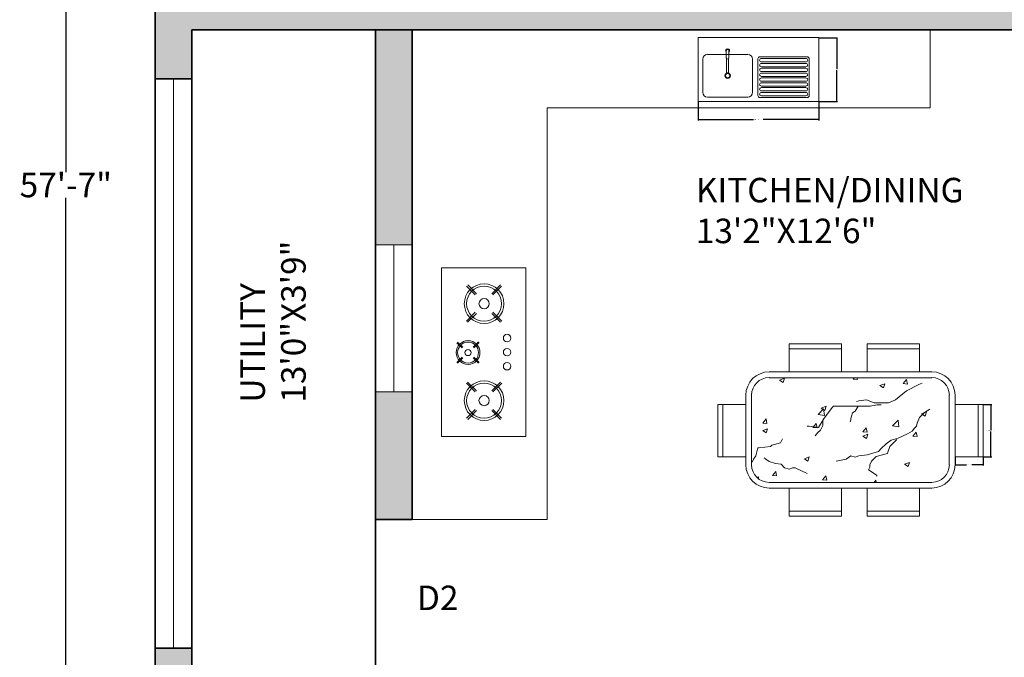
# Model space of a CAD drawing. Units: inches. Extents: x -9 to 505, y -680 to 48.
# Tile 2 of 17: x -6 to 235, y -450 to -293. Entities that reach past the tile are written whole.
import ezdxf

# ---------------------------------------------------------------- set-up
doc = ezdxf.new("R2010")
doc.units = ezdxf.units.IN
doc.header["$MEASUREMENT"] = 0
for name, color, linetype, lineweight in [('A-ANNO-DIMS', 2, 'Continuous', 18), ('A-ANNO-TEXT', 7, 'Continuous', 18), ('A-AREA-IDEN', 7, 'Continuous', 18), ('A-EQPM', 8, 'Continuous', 18), ('A-FLOR-CASE', 8, 'Continuous', 18), ('A-FLOR-FIXT', 9, 'Continuous', 18), ('A-FLOR-HRAL', 4, 'Continuous', 18), ('A-FURN', 8, 'Continuous', 18), ('A-GLAZ', 4, 'Continuous', 18), ('A-WALL', 7, 'Continuous', 35), ('A-WALL-PATT', 251, 'Continuous', 13), ('S-CONC', 7, 'Continuous', 35), ('S-CONC-PATT', 18, 'Continuous', 13)]:
    doc.layers.add(name, color=color, linetype=linetype, lineweight=lineweight)
doc.styles.get("Standard").update_dxf_attribs({"font": 'arial.ttf'})
doc.dimstyles.get("Standard").update_dxf_attribs({"dimtxt": 0.18, "dimasz": 0.18, "dimexe": 0.18, "dimexo": 0.0625, "dimgap": 0.09, "dimtad": 0, "dimtih": 1, "dimtoh": 1, "dimdec": 0, "dimzin": 0, "dimdsep": 46, "dimlunit": 3, "dimtxsty": 'Standard', "dimcen": 0.09, "dimadec": 0, "dimazin": 0, "dimtfac": 1, "dimtdec": 0, "dimtofl": 0, "dimtmove": 0, "dimatfit": 3, "dimfxl": 1, "dimtolj": 1, "dimtzin": 0, "dimarcsym": 0})

# ---------------------------------------------------------------- blocks, each defined once
blk = doc.blocks.new('*D3')
at = {"layer": 'A-ANNO-DIMS', "color": 0, "lineweight": -2, "transparency": 16777216}
for p, q in [((27.2, 11.5), (5.16, 11.5)), ((5.34, 11.32), (5.34, -330.86)), ((5.34, -679.32), (5.34, -337.14)), ((27.2, -679.5), (5.16, -679.5))]:
    blk.add_line(p, q, dxfattribs=at)
at = {"layer": 'A-ANNO-DIMS', "color": 0, "transparency": 16777216}
for points in [[(5.31, 11.32), (5.37, 11.32), (5.34, 11.5)], [(5.31, -679.32), (5.37, -679.32), (5.34, -679.5)]]:
    blk.add_solid(points, dxfattribs=at)
at = {"layer": 'Defpoints', "color": 0, "transparency": 16777216}
for p in [(27.26, 11.5), (5.34, -679.5), (27.26, -679.5)]:
    blk.add_point(p, dxfattribs=at)
at = {"layer": 'A-ANNO-DIMS', "color": 0, "transparency": 16777216, "insert": (5.34, -334), "char_height": 6, "attachment_point": 5}
blk.add_mtext('\\A1;57\'-7"', dxfattribs=at)
blk = doc.blocks.new('WIN-36')
for p, q in [((0, 36), (0, 0)), ((9, 36), (0, 36)), ((4.5, 36), (4.5, 2.23)), ((9, 0), (9, 36)), ((0, 0), (9, 0)), ((4.5, 2.23), (4.5, 0))]:
    blk.add_line(p, q)
blk = doc.blocks.new('SINK-SINGLE-DRAINBOARD')
for p, q in [((0, 0), (0, 15.65)), ((0, 15.65), (29.6, 15.65)), ((29.6, 0), (29.6, 15.65)), ((1.13, 10.39), (1.13, 2.25)), ((7.43, 11.55), (2.3, 11.55)), ((12.19, 11.55), (7.57, 11.55)), ((13.36, 2.25), (13.36, 10.39)), ((14.68, 10.42), (14.68, 1.51)), ((26.71, 10.96), (15.22, 10.96)), ((20.97, 10.52), (15.55, 10.52)), ((20.97, 9.72), (15.55, 9.72)), ((20.97, 10.52), (26.39, 10.52)), ((20.97, 9.72), (26.39, 9.72)), ((27.25, 10.42), (27.25, 1.51)), ((20.97, 9.34), (15.55, 9.34)), ((20.97, 8.53), (15.55, 8.53)), ((20.97, 8.15), (15.55, 8.15)), ((20.97, 7.34), (15.55, 7.34)), ((20.97, 9.34), (26.39, 9.34)), ((20.97, 8.53), (26.39, 8.53)), ((20.97, 8.15), (26.39, 8.15)), ((20.97, 7.34), (26.39, 7.34)), ((20.97, 6.96), (15.55, 6.96)), ((20.97, 6.15), (15.55, 6.15)), ((20.97, 5.77), (15.55, 5.77)), ((20.97, 4.96), (15.55, 4.96)), ((20.97, 6.96), (26.39, 6.96)), ((20.97, 6.15), (26.39, 6.15)), ((20.97, 5.77), (26.39, 5.77)), ((20.97, 4.96), (26.39, 4.96)), ((20.97, 4.58), (15.55, 4.58)), ((20.97, 3.78), (15.55, 3.78)), ((20.97, 3.4), (15.55, 3.4)), ((20.97, 2.59), (15.55, 2.59)), ((20.97, 4.58), (26.39, 4.58)), ((20.97, 3.78), (26.39, 3.78)), ((20.97, 3.4), (26.39, 3.4)), ((20.97, 2.59), (26.39, 2.59)), ((2.3, 1.09), (12.19, 1.09)), ((15.22, 0.97), (26.71, 0.97)), ((20.97, 2.21), (15.55, 2.21)), ((20.97, 1.4), (15.55, 1.4)), ((20.97, 2.21), (26.39, 2.21)), ((20.97, 1.4), (26.39, 1.4)), ((0, 0), (29.6, 0))]:
    blk.add_line(p, q)
for points in [[(6.92, 12.46), (6.92, 10.68)], [(7.57, 12.46), (7.57, 10.68)], [(7, 10.48), (7, 7.2)], [(7.49, 10.48), (7.49, 7.2)]]:
    blk.add_lwpolyline(points)
for radius in [0.674, 0.54]:
    blk.add_circle((7.25, 6.32), radius)
for centre, radius, start, end in [((7.25, 12.46), 0.485, 311.9018, 228.0982), ((7.25, 12.46), 0.324, 0, 180), ((2.3, 10.39), 1.17, 90, 180), ((7.25, 10.69), 0.324, 182.2198, 357.7802), ((12.19, 10.39), 1.17, 0, 90), ((15.22, 10.42), 0.54, 90, 180), ((15.55, 9.99), 0.54, 90, 165.5097), ((15.55, 10.26), 0.54, 194.4903, 270), ((26.39, 9.99), 0.54, 14.4903, 90), ((26.39, 10.26), 0.54, 270, 345.5097), ((26.71, 10.42), 0.54, 0, 90), ((15.55, 8.8), 0.54, 90, 165.5097), ((15.55, 9.07), 0.54, 194.4903, 270), ((15.55, 7.61), 0.54, 90, 165.5097), ((15.55, 7.88), 0.54, 194.4903, 270), ((26.39, 8.8), 0.54, 14.4903, 90), ((26.39, 9.07), 0.54, 270, 345.5097), ((26.39, 7.61), 0.54, 14.4903, 90), ((26.39, 7.88), 0.54, 270, 345.5097), ((7.25, 7.18), 0.244, 174.9463, 5.0537), ((15.55, 6.42), 0.54, 90, 165.5097), ((15.55, 6.69), 0.54, 194.4903, 270), ((15.55, 5.23), 0.54, 90, 165.5097), ((15.55, 5.5), 0.54, 194.4903, 270), ((26.39, 6.42), 0.54, 14.4903, 90), ((26.39, 6.69), 0.54, 270, 345.5097), ((26.39, 5.23), 0.54, 14.4903, 90), ((26.39, 5.5), 0.54, 270, 345.5097), ((15.55, 4.05), 0.54, 90, 165.5097), ((15.55, 4.32), 0.54, 194.4903, 270), ((15.55, 2.86), 0.54, 90, 165.5097), ((15.55, 3.13), 0.54, 194.4903, 270), ((26.39, 4.05), 0.54, 14.4903, 90), ((26.39, 4.32), 0.54, 270, 345.5097), ((26.39, 2.86), 0.54, 14.4903, 90), ((26.39, 3.13), 0.54, 270, 345.5097), ((2.3, 2.25), 1.17, 180, 270), ((12.19, 2.25), 1.17, 270, 0), ((15.22, 1.51), 0.54, 180, 270), ((15.55, 1.67), 0.54, 90, 165.5097), ((15.55, 1.94), 0.54, 194.4903, 270), ((26.39, 1.67), 0.54, 14.4903, 90), ((26.39, 1.94), 0.54, 270, 345.5097), ((26.71, 1.51), 0.54, 270, 0)]:
    blk.add_arc(centre, radius, start, end)
blk = doc.blocks.new('CHAIR-DINING-RECTANGULAR')
for p, q in [((6.87, 12.83), (0, 12.83)), ((5.62, 12.83), (5.62, 0)), ((6.87, 0), (6.87, 12.83)), ((0, 0), (6.87, 0))]:
    blk.add_line(p, q)
blk = doc.blocks.new('*D28')
at = {"layer": 'A-ANNO-DIMS', "color": 0, "lineweight": -2, "transparency": 16777216}
for p, q in [((160.34, -313.6), (160.34, -318.15)), ((189.94, -313.6), (189.94, -318.15)), ((160.52, -317.97), (173.96, -317.97)), ((189.76, -317.97), (176.32, -317.97))]:
    blk.add_line(p, q, dxfattribs=at)
at = {"layer": 'A-ANNO-DIMS', "color": 0, "transparency": 16777216}
for points in [[(160.52, -317.94), (160.52, -318), (160.34, -317.97)], [(189.76, -317.94), (189.76, -318), (189.94, -317.97)]]:
    blk.add_solid(points, dxfattribs=at)
at = {"layer": 'Defpoints', "color": 0, "transparency": 16777216}
for p in [(160.34, -313.53), (189.94, -313.53), (189.94, -317.97)]:
    blk.add_point(p, dxfattribs=at)
at = {"layer": 'A-ANNO-DIMS', "color": 0, "transparency": 16777216, "insert": (175.14, -317.97), "char_height": 0.18, "attachment_point": 5}
blk.add_mtext('\\A1;SINK 2\'-5 1/2" TYP.', dxfattribs=at)
blk = doc.blocks.new('*D29')
at = {"layer": 'A-ANNO-DIMS', "color": 0, "lineweight": -2, "transparency": 16777216}
for p, q in [((190, -297.89), (194.56, -297.89)), ((194.38, -298.07), (194.38, -305.53)), ((194.38, -313.35), (194.38, -305.89)), ((190, -313.53), (194.56, -313.53))]:
    blk.add_line(p, q, dxfattribs=at)
at = {"layer": 'A-ANNO-DIMS', "color": 0, "transparency": 16777216}
for points in [[(194.35, -298.07), (194.41, -298.07), (194.38, -297.89)], [(194.35, -313.35), (194.41, -313.35), (194.38, -313.53)]]:
    blk.add_solid(points, dxfattribs=at)
at = {"layer": 'Defpoints', "color": 0, "transparency": 16777216}
for p in [(189.94, -297.89), (194.38, -297.89), (189.94, -313.53)]:
    blk.add_point(p, dxfattribs=at)
at = {"layer": 'A-ANNO-DIMS', "color": 0, "transparency": 16777216, "insert": (194.38, -305.71), "char_height": 0.18, "attachment_point": 5}
blk.add_mtext('\\A1;1\'-3 1/2" TYP.', dxfattribs=at)
blk = doc.blocks.new('*D40')
at = {"layer": 'A-ANNO-DIMS', "color": 0, "lineweight": -2, "transparency": 16777216}
for p, q in [((230.29, -387.8), (232.33, -387.8)), ((232.15, -387.98), (232.15, -394.03)), ((232.15, -400.45), (232.15, -394.4)), ((230.29, -400.63), (232.33, -400.63))]:
    blk.add_line(p, q, dxfattribs=at)
at = {"layer": 'A-ANNO-DIMS', "color": 0, "transparency": 16777216}
for points in [[(232.12, -387.98), (232.18, -387.98), (232.15, -387.8)], [(232.12, -400.45), (232.18, -400.45), (232.15, -400.63)]]:
    blk.add_solid(points, dxfattribs=at)
at = {"layer": 'Defpoints', "color": 0, "transparency": 16777216}
for p in [(230.23, -387.8), (232.15, -387.8), (230.23, -400.63)]:
    blk.add_point(p, dxfattribs=at)
at = {"layer": 'A-ANNO-DIMS', "color": 0, "transparency": 16777216, "insert": (232.15, -394.21), "char_height": 0.18, "attachment_point": 5}
blk.add_mtext('\\A1;SIDE CHAIR 1\'-1" TYP.', dxfattribs=at)
blk = doc.blocks.new('*D41')
at = {"layer": 'A-ANNO-DIMS', "color": 0, "lineweight": -2, "transparency": 16777216}
for p, q in [((223.36, -400.69), (223.36, -402.73)), ((230.23, -400.69), (230.23, -402.73)), ((223.54, -402.55), (226.15, -402.55)), ((230.05, -402.55), (227.43, -402.55))]:
    blk.add_line(p, q, dxfattribs=at)
at = {"layer": 'A-ANNO-DIMS', "color": 0, "transparency": 16777216}
for points in [[(223.54, -402.52), (223.54, -402.58), (223.36, -402.55)], [(230.05, -402.52), (230.05, -402.58), (230.23, -402.55)]]:
    blk.add_solid(points, dxfattribs=at)
at = {"layer": 'Defpoints', "color": 0, "transparency": 16777216}
for p in [(223.36, -400.63), (230.23, -400.63), (230.23, -402.55)]:
    blk.add_point(p, dxfattribs=at)
at = {"layer": 'A-ANNO-DIMS', "color": 0, "transparency": 16777216, "insert": (226.79, -402.55), "char_height": 0.18, "attachment_point": 5}
blk.add_mtext('\\A1;0\'-7" TYP.', dxfattribs=at)

msp = doc.modelspace()

# ---------------------------------------------------------------- hatches: boundary and pattern name
at = {"layer": 'A-WALL-PATT'}
h = msp.add_hatch(color=256, dxfattribs=at)
h.dxf.hatch_style = 1
h.paths.add_polyline_path([(101.64, 11.5), (48.26, 11.5), (48.26, 2.5), (72.26, 2.5), (72.26, -21.25), (81.26, -21.25), (81.26, 2.5), (101.64, 2.5)])
h.paths.add_polyline_path([(36.26, 2.5), (27.26, 2.5), (27.26, -6.92), (36.26, -6.92)])
h.paths.add_polyline_path([(81.26, -57.25), (72.26, -57.25), (72.26, -75.5), (81.26, -75.5)])
h.paths.add_polyline_path([(162.76, 11.5), (137.64, 11.5), (137.64, 2.5), (162.76, 2.5)])
h.paths.add_polyline_path([(179.26, 2.5), (174.76, 2.5), (174.76, -75.5), (179.26, -75.5), (179.26, -54.5), (229.51, -54.5), (229.51, -45.5), (179.26, -45.5)])
h.paths.add_polyline_path([(382.26, -45.5), (332.26, -45.5), (332.26, 2.5), (327.76, 2.5), (327.76, -45.5), (277.51, -45.5), (277.51, -54.5), (327.76, -54.5), (327.76, -111.5), (332.26, -111.5), (332.26, -54.5), (382.26, -54.5)])
h.paths.add_polyline_path([(332.26, -128), (327.76, -128), (327.76, -207), (332.26, -207)])
h.paths.add_polyline_path([(124.76, -111.5), (36.26, -111.5), (36.26, -116), (120.26, -116), (120.26, -168.5), (179.26, -168.5), (179.26, -164), (124.76, -164)])
h.paths.add_polyline_path([(96.26, -164), (36.26, -164), (36.26, -152), (27.26, -152), (27.26, -208.88), (36.26, -208.88), (36.26, -168.5), (96.26, -168.5)])
h.paths.add_polyline_path([(36.26, -244.88), (27.26, -244.88), (27.26, -287), (36.26, -287)])
h.paths.add_polyline_path([(179.26, -204.5), (174.76, -204.5), (174.76, -287), (179.26, -287)])
h.paths.add_polyline_path([(257.26, -296), (248.26, -296), (248.26, -446), (269.26, -446), (269.26, -437), (257.26, -437)])
h.paths.add_polyline_path([(90.26, -296), (81.26, -296), (81.26, -348.67), (90.26, -348.67)])
h.paths.add_polyline_path([(90.26, -384.67), (81.26, -384.67), (81.26, -416), (90.26, -416)])
h.paths.add_polyline_path([(170.26, -452), (36.26, -452), (36.26, -456.5), (165.76, -456.5), (165.76, -504.5), (165.13, -504.5), (165.13, -509), (170.26, -509)])
h.paths.add_polyline_path([(141.76, -504.5), (36.26, -504.5), (36.26, -492.5), (27.26, -492.5), (27.26, -565.96), (36.26, -565.96), (36.26, -509), (141.76, -509)])
h.paths.add_polyline_path([(36.26, -601.96), (27.26, -601.96), (27.26, -658.5), (36.26, -658.5)])
h.paths.add_polyline_path([(170.26, -670.5), (170.26, -634.5), (222.76, -634.5), (222.76, -625.5), (165.76, -625.5), (165.76, -670.5), (36.26, -670.5), (36.26, -679.5), (170.26, -679.5)])
h.paths.add_polyline_path([(332.26, -616.5), (433.89, -616.5), (433.89, -612), (332.26, -612), (332.26, -610.56), (327.76, -610.56), (327.76, -625.5), (270.76, -625.5), (270.76, -634.5), (327.76, -634.5), (327.76, -658.5), (332.26, -658.5)])
h.paths.add_polyline_path([(459.76, -670.5), (336.76, -670.5), (336.76, -679.5), (459.76, -679.5)])
h.paths.add_polyline_path([(468.76, -545.74), (459.76, -545.74), (459.76, -612), (457.89, -612), (457.89, -616.5), (459.76, -616.5), (459.76, -658.5), (468.76, -658.5)])
h.paths.add_polyline_path([(332.26, -446), (327.76, -446), (327.76, -574.56), (332.26, -574.56)])
h.paths.add_polyline_path([(327.76, -437), (305.26, -437), (305.26, -446), (327.76, -446)])
h.paths.add_polyline_path([(459.76, -437), (348.76, -437), (348.76, -446), (459.76, -446)])
h.paths.add_polyline_path([(468.76, -458), (459.76, -458), (459.76, -509.74), (468.76, -509.74)])
h.paths.add_polyline_path([(468.76, -365), (459.76, -365), (459.76, -437), (468.76, -437)])
h.paths.add_polyline_path([(468.76, -299.6), (459.76, -299.6), (459.76, -344), (468.76, -344)])
h.paths.add_polyline_path([(468.76, -184.74), (459.76, -184.74), (459.76, -231), (401.26, -231), (401.26, -235.5), (459.76, -235.5), (459.76, -275.6), (468.76, -275.6)])
h.paths.add_polyline_path([(390.76, -356), (342.76, -356), (342.76, -365), (390.76, -365)])
h.paths.add_polyline_path([(459.76, -356), (405.76, -356), (405.76, -365), (459.76, -365)])
h.paths.add_polyline_path([(405.76, -296), (396.76, -296), (396.76, -356), (405.76, -356)])
h.paths.add_polyline_path([(336.76, -296), (327.76, -296), (327.76, -356), (336.76, -356)])
h.paths.add_polyline_path([(468.76, -9.5), (459.76, -9.5), (459.76, -45.5), (418.26, -45.5), (418.26, -54.5), (468.76, -54.5)])
h.paths.add_polyline_path([(468.76, -54.5), (459.76, -54.5), (459.76, -111.5), (468.76, -111.5)])
h.paths.add_polyline_path([(468.76, -128), (459.76, -128), (459.76, -148.74), (468.76, -148.74)])
at = {"layer": 'S-CONC-PATT'}
h = msp.add_hatch(color=256, dxfattribs=at)
h.dxf.hatch_style = 1
h.paths.add_polyline_path([(269.26, -296), (269.26, -287), (27.26, -287), (27.26, -308), (36.26, -308), (36.26, -296)])
h = msp.add_hatch(color=256, dxfattribs=at)
h.dxf.hatch_style = 1
h.paths.add_polyline_path([(36.26, -447.5), (27.26, -447.5), (27.26, -468.5), (36.26, -468.5), (36.26, -456.5), (36.26, -452)])

# ---------------------------------------------------------------- linework, layer by layer
at = {"layer": 'A-EQPM'}
for p, q in [((97.43, -354.27), (97.43, -395.65)), ((118.12, -354.27), (97.43, -354.27)), ((118.12, -395.65), (118.12, -354.27)), ((105.73, -360.93), (103.58, -358.78)), ((106.02, -360.64), (103.86, -358.49)), ((109.74, -360.64), (111.89, -358.49)), ((110.02, -360.93), (112.18, -358.78)), ((105.71, -365.2), (103.54, -367.34)), ((106, -365.49), (103.83, -367.63)), ((109.75, -365.49), (111.93, -367.63)), ((110.04, -365.2), (112.21, -367.34)), ((102.49, -373.94), (101.2, -372.65)), ((102.66, -373.77), (101.37, -372.48)), ((105.23, -373.76), (106.51, -372.46)), ((105.4, -373.93), (106.68, -372.63)), ((102.49, -376.17), (101.2, -377.47)), ((102.66, -376.34), (101.37, -377.64)), ((105.23, -376.35), (106.51, -377.66)), ((105.4, -376.18), (106.68, -377.49)), ((105.71, -384.71), (103.54, -382.58)), ((106, -384.42), (103.83, -382.29)), ((109.75, -384.42), (111.93, -382.29)), ((110.04, -384.71), (112.21, -382.58)), ((105.73, -388.99), (103.58, -391.14)), ((106.02, -389.27), (103.86, -391.43)), ((109.74, -389.27), (111.89, -391.43)), ((110.02, -388.99), (112.18, -391.14)), ((97.43, -395.65), (118.12, -395.65))]:
    msp.add_line(p, q, dxfattribs=at)
for centre, radius in [((107.88, -363.08), 4.86), ((107.88, -363.08), 4.28), ((107.88, -363.08), 1.25), ((113.52, -371.51), 0.919), ((103.95, -375.06), 2.92), ((103.95, -375.06), 2.57), ((113.52, -374.96), 0.919), ((103.95, -375.06), 0.752), ((113.52, -378.41), 0.919), ((107.88, -386.84), 4.86), ((107.88, -386.84), 4.28), ((107.88, -386.84), 1.25)]:
    msp.add_circle(centre, radius, dxfattribs=at)
at = {"layer": 'A-FLOR-CASE'}
for p, q in [((217.26, -315.07), (217.26, -296)), ((123.35, -416), (123.35, -315.07)), ((123.35, -315.07), (217.26, -315.07)), ((90.26, -416), (123.35, -416))]:
    msp.add_line(p, q, dxfattribs=at)
at = {"layer": 'A-FLOR-HRAL'}
for p, q in [((36.26, -308), (27.26, -308)), ((27.26, -308), (27.26, -447.5)), ((31.76, -308), (31.76, -447.5)), ((36.26, -447.5), (36.26, -308)), ((36.26, -447.5), (27.26, -447.5))]:
    msp.add_line(p, q, dxfattribs=at)
at = {"layer": 'A-FURN'}
for p, q in [((217.66, -379.79), (177.75, -379.79)), ((177.75, -381.22), (217.66, -381.22)), ((180.34, -381.79), (181.54, -381.33)), ((181.19, -382.36), (181.54, -381.33)), ((198.37, -381.61), (198.7, -381.22)), ((199.39, -381.7), (199.3, -381.22)), ((180.34, -381.79), (181.19, -382.36)), ((198.37, -381.61), (199.39, -381.7)), ((204.92, -383.16), (206.12, -382.7)), ((204.92, -383.16), (205.77, -383.73)), ((205.77, -383.73), (206.12, -382.7)), ((210.63, -382.68), (211.46, -381.7)), ((210.63, -382.68), (211.66, -382.77)), ((214.5, -382.91), (211.4, -384.45)), ((211.66, -382.77), (211.46, -381.7)), ((215.27, -382.6), (214.5, -382.91)), ((172.05, -385.49), (172.05, -402.59)), ((173.47, -402.59), (173.47, -385.49)), ((211.4, -384.45), (208.76, -386.62)), ((221.93, -385.49), (221.93, -402.59)), ((223.36, -402.59), (223.36, -385.49)), ((190.55, -388.67), (191.75, -388.21)), ((193.26, -388.48), (191.25, -391.11)), ((191.4, -389.25), (191.75, -388.21)), ((193.57, -388.17), (193.26, -388.48)), ((202.56, -388.17), (193.57, -388.17)), ((199.31, -388.63), (198.85, -389.4)), ((199.77, -386.93), (199.15, -387.08)), ((199.62, -388.16), (199.31, -388.63)), ((201.63, -386.62), (199.77, -386.93)), ((203.49, -387.39), (201.63, -386.62)), ((204.27, -387.86), (202.56, -388.17)), ((207.06, -387.39), (203.49, -387.39)), ((205.2, -387.86), (204.27, -387.86)), ((208.76, -386.62), (207.06, -387.39)), ((189.78, -390.23), (191.11, -388.84)), ((189.78, -390.23), (191.3, -390.46)), ((190.55, -388.67), (191.4, -389.25)), ((191.3, -390.46), (191.11, -388.84)), ((197.92, -390.64), (197.76, -391.26)), ((198.23, -389.87), (197.92, -390.64)), ((198.85, -389.4), (198.23, -389.87)), ((214.65, -390.95), (214.03, -392.35)), ((215.89, -389.72), (214.65, -390.95)), ((215.13, -390.04), (216.33, -389.58)), ((215.13, -390.04), (215.98, -390.62)), ((217.13, -388.94), (215.89, -389.72)), ((215.98, -390.62), (216.33, -389.58)), ((176.21, -392.33), (177.03, -391.34)), ((176.21, -392.33), (177.23, -392.42)), ((177.23, -392.42), (177.03, -391.34)), ((187.53, -393.12), (187.07, -393.12)), ((189.85, -393.43), (187.53, -393.12)), ((188.47, -393.4), (189.3, -392.42)), ((188.47, -393.4), (189.5, -393.49)), ((189.5, -393.49), (189.3, -392.42)), ((191.25, -391.11), (189.85, -393.43)), ((190.94, -392.97), (190.32, -394.05)), ((190.94, -391.57), (190.94, -392.97)), ((197.76, -391.57), (197.61, -392.03)), ((197.76, -391.26), (197.76, -391.57)), ((208.03, -393.06), (209.36, -391.67)), ((208.03, -393.06), (209.55, -393.29)), ((209.55, -393.29), (209.36, -391.67)), ((213.88, -393.12), (213.41, -393.59)), ((214.03, -392.35), (213.88, -393.12)), ((176.18, -394.19), (177.38, -393.73)), ((176.18, -394.19), (177.03, -394.76)), ((177.03, -394.76), (177.38, -393.73)), ((189.7, -394.67), (189.08, -395.44)), ((190.32, -394.05), (189.7, -394.67)), ((200.74, -394.47), (201.57, -393.49)), ((200.74, -394.47), (201.76, -394.56)), ((200.76, -395.56), (201.95, -395.1)), ((200.76, -395.56), (201.61, -396.13)), ((201.76, -394.56), (201.57, -393.49)), ((201.61, -396.13), (201.96, -395.1)), ((211.71, -394.98), (209.38, -396.06)), ((212.79, -394.36), (211.71, -394.98)), ((213.41, -393.59), (212.79, -394.36)), ((213.01, -395.55), (213.83, -394.56)), ((213.01, -395.55), (214.03, -395.64)), ((214.03, -395.64), (213.83, -394.56)), ((175.29, -398.38), (178.08, -398.08)), ((178.08, -398.08), (178.39, -397.77)), ((178.39, -397.77), (180.56, -397.15)), ((180.56, -397.15), (181.02, -396.22)), ((206.44, -397.46), (205.2, -398.54)), ((207.68, -396.53), (206.44, -397.46)), ((207.37, -398.08), (206.9, -399.47)), ((208.45, -396.99), (207.37, -398.08)), ((209.38, -396.06), (207.68, -396.53)), ((209.07, -396.37), (208.45, -396.99)), ((173.89, -401.17), (174.51, -400.4)), ((174.51, -400.4), (174.98, -398.38)), ((174.98, -398.38), (175.29, -398.38)), ((186.39, -401.07), (187.58, -400.61)), ((187.24, -401.65), (187.58, -400.61)), ((197.76, -400.4), (196.67, -401.17)), ((198.84, -400.71), (197.76, -400.4)), ((199.77, -400.4), (198.84, -400.71)), ((201.79, -400.09), (199.77, -400.4)), ((204.58, -399.31), (201.79, -400.09)), ((203.96, -400.55), (202.87, -401.64)), ((206.75, -399.78), (203.96, -400.55)), ((205.2, -398.54), (204.58, -399.31)), ((206.9, -399.47), (206.75, -399.78)), ((173.58, -401.94), (173.89, -401.17)), ((176.99, -401.17), (176.53, -400.86)), ((177.77, -401.78), (176.99, -401.17)), ((179.32, -402.25), (177.77, -401.78)), ((180.71, -402.4), (179.32, -402.25)), ((181.49, -403.33), (180.71, -402.4)), ((186.39, -401.07), (187.24, -401.65)), ((196.67, -401.17), (194.19, -401.64)), ((202.87, -401.64), (202.41, -402.56)), ((202.41, -402.56), (202.41, -403.18)), ((210.97, -402.44), (212.16, -401.98)), ((210.97, -402.44), (211.82, -403.02)), ((211.82, -403.02), (212.16, -401.98)), ((174.88, -405.76), (175.13, -405.5)), ((175.19, -406.02), (175.13, -405.5)), ((178.58, -405.19), (179.4, -404.21)), ((178.58, -405.19), (179.6, -405.28)), ((179.6, -405.28), (179.4, -404.21)), ((182.73, -403.64), (181.49, -403.33)), ((183.5, -403.33), (182.73, -403.64)), ((184.12, -403.33), (183.5, -403.33)), ((187.07, -404.73), (184.12, -403.33)), ((190.85, -406.26), (191.67, -405.28)), ((191.87, -406.35), (191.67, -405.28)), ((202.41, -403.18), (202.1, -403.8)), ((202.1, -403.8), (203.96, -405.04)), ((203.96, -405.04), (204.27, -405.35)), ((217.66, -406.87), (177.75, -406.87)), ((190.85, -406.26), (191.87, -406.35)), ((203.51, -406.87), (203.94, -406.36)), ((204.03, -406.87), (203.94, -406.36)), ((177.75, -408.3), (217.66, -408.3))]:
    msp.add_line(p, q, dxfattribs=at)
for centre, radius, start, end in [((177.75, -385.49), 5.7, 90, 180), ((177.75, -385.49), 4.28, 90, 180), ((217.66, -385.49), 5.7, 0, 90), ((217.66, -385.49), 4.28, 0, 90), ((177.75, -402.59), 5.7, 180, 270), ((177.75, -402.59), 4.28, 180, 270), ((217.66, -402.59), 4.28, 270, 0), ((217.66, -402.59), 5.7, 270, 0)]:
    msp.add_arc(centre, radius, start, end, dxfattribs=at)
at = {"layer": 'A-WALL'}
for p, q in [((27.26, 11.5), (27.26, -679.5)), ((36.26, -296), (405.76, -296)), ((36.26, -296), (36.26, -452)), ((81.26, -296), (81.26, -416)), ((90.26, -296), (90.26, -416)), ((90.26, -416), (81.26, -416)), ((81.26, -416), (81.26, -452))]:
    msp.add_line(p, q, dxfattribs=at)
at = {"layer": 'S-CONC'}
for p, q in [((36.26, -308), (27.26, -308)), ((36.26, -447.5), (27.26, -447.5))]:
    msp.add_line(p, q, dxfattribs=at)

# ---------------------------------------------------------------- block references
at = {"layer": 'A-FLOR-FIXT'}
msp.add_blockref('SINK-SINGLE-DRAINBOARD', (160.34, -313.53), dxfattribs=at)
at = {"layer": 'A-FURN'}
for p, rotation in [((195.51, -379.79), 89.99999998729292), ((214.61, -379.79), 89.99999998729254), ((172.05, -387.8), 180), ((182.68, -408.3), 269.999999988474), ((201.78, -408.3), 269.9999999884739)]:
    msp.add_blockref('CHAIR-DINING-RECTANGULAR', p, dxfattribs=dict(at, rotation=rotation))
msp.add_blockref('CHAIR-DINING-RECTANGULAR', (223.36, -400.63), dxfattribs=at)
at = {"layer": 'A-GLAZ'}
msp.add_blockref('WIN-36', (81.26, -384.67), dxfattribs=at)

# ---------------------------------------------------------------- texts
at = {"layer": 'A-ANNO-TEXT', "insert": (91.42, -432.18), "char_height": 6, "attachment_point": 1}
msp.add_mtext_dynamic_manual_height_columns('D2', width=1.6434, gutter_width=1, heights=[0], dxfattribs=at)
at = {"layer": 'A-AREA-IDEN', "insert": (159.8, -332.25), "char_height": 6, "attachment_point": 1}
msp.add_mtext('KITCHEN/DINING\\P13\'2"X12\'6"', dxfattribs=at)
at = {"layer": 'A-AREA-IDEN', "insert": (48.14, -387.34), "char_height": 6, "attachment_point": 1, "rotation": 90}
msp.add_mtext('UTILITY\\P13\'0"X3\'9"', dxfattribs=at)

# ---------------------------------------------------------------- dimensions: what is measured, and where the dimension line sits
at = {"layer": 'A-ANNO-DIMS'}
dim = msp.add_linear_dim(base=(5.34, -679.5), p1=(27.26, 11.5), p2=(27.26, -679.5), angle=90, dimstyle='Standard', override={"dimtxt": 6, "dimclrd": 0, "dimclre": 0, "dimclrt": 0}, dxfattribs=at)
dim.commit()
dim.dimension.update_dxf_attribs({"geometry": '*D3', "text_midpoint": (5.34, -334)})
for base, p1, p2, text, picture, middle in [((194.38, -297.89), (189.94, -313.53), (189.94, -297.89), '<> TYP.', '*D29', (194.38, -305.71)), ((232.15, -387.8), (230.23, -400.63), (230.23, -387.8), 'SIDE CHAIR <> TYP.', '*D40', (232.15, -394.21))]:
    dim = msp.add_linear_dim(base=base, p1=p1, p2=p2, angle=90, text=text, dimstyle='Standard', override={"dimdec": 1, "dimlfac": 1, "dimrnd": 0, "dimzin": 1, "dimdsep": 46, "dimlunit": 4, "dimfrac": 2}, dxfattribs=at)
    dim.commit()
    dim.dimension.update_dxf_attribs({"geometry": picture, "text_midpoint": middle})
for base, p1, p2, text, picture, middle in [((189.94, -317.97), (160.34, -313.53), (189.94, -313.53), 'SINK <> TYP.', '*D28', (175.14, -317.97)), ((230.23, -402.55), (223.36, -400.63), (230.23, -400.63), '<> TYP.', '*D41', (226.79, -402.55))]:
    dim = msp.add_linear_dim(base=base, p1=p1, p2=p2, text=text, dimstyle='Standard', override={"dimdec": 1, "dimlfac": 1, "dimrnd": 0, "dimzin": 1, "dimdsep": 46, "dimlunit": 4, "dimfrac": 2}, dxfattribs=at)
    dim.commit()
    dim.dimension.update_dxf_attribs({"geometry": picture, "text_midpoint": middle})

doc.saveas('drawing.dxf')
